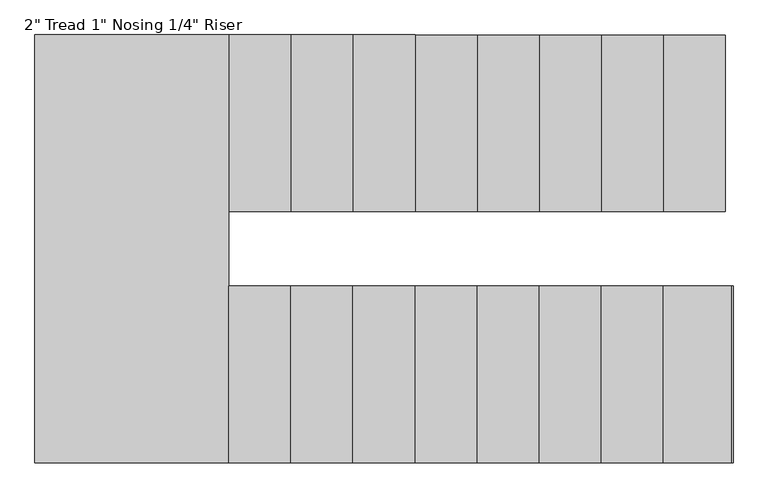
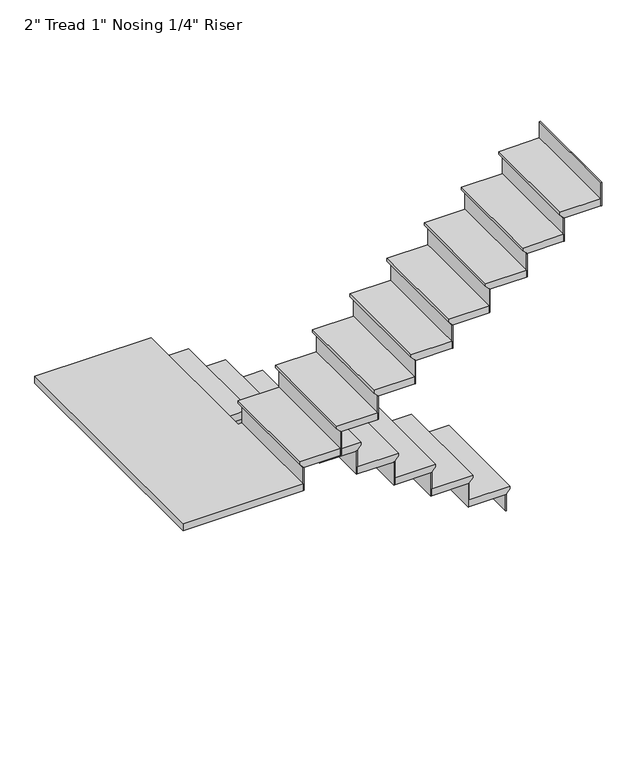
"""IFC4 building model written with IfcOpenShell, lengths in millimetres: stair flight geometry."""

from ifc_helpers import new_model, si_unit, origin, place, context, project, spatial, faceted_brep, source, transform, mapped, element, save


def stair_flight_1a1858fe(model_context):
    return source(origin(), model_context, "Body", "Brep", [
        faceted_brep([(-2118.1728655, 1192.5797121, 3196.8722222), (-2118.1728655, 1192.5797121, 3215.9222222), (-2118.1728655, 468.6797121, 3215.9222222), (-2118.1728655, 468.6797121, 3196.8722222), (-2143.5728655, 1192.5797121, 3171.4722222), (-2143.5728655, 468.6797121, 3171.4722222), (-2397.5728655, 1192.5797121, 3215.9222222), (-2397.5728655, 468.6797121, 3215.9222222), (-2143.5728655, 468.6797121, 3165.1222222), (-2397.5728655, 468.6797121, 3165.1222222), (-2397.5728655, 1192.5797121, 3165.1222222), (-2143.5728655, 1192.5797121, 3165.1222222)], [[[0, 1, 2, 3]], [[4, 0, 3, 5]], [[2, 1, 6, 7]], [[8, 9, 10, 11]], [[2, 7, 9, 8, 5, 3]], [[8, 11, 4, 5]], [[6, 1, 0, 4, 11, 10]], [[7, 6, 10, 9]]]),
        faceted_brep([(-2143.5728655, 1192.5797121, 3165.1222222), (-2143.5728655, 1192.5797121, 3048.0), (-2149.9228655, 1192.5797121, 3048.0), (-2149.9228655, 1192.5797121, 3165.1222222), (-2143.5728655, 468.6797121, 3165.1222222), (-2149.9228655, 468.6797121, 3165.1222222), (-2149.9228655, 468.6797121, 3048.0), (-2143.5728655, 468.6797121, 3048.0)], [[[0, 1, 2, 3]], [[4, 5, 6, 7]], [[1, 0, 4, 7]], [[2, 1, 7, 6]], [[3, 2, 6, 5]], [[0, 3, 5, 4]]]),
        faceted_brep([(-2397.5728655, 1192.5797121, 3333.0444444), (-2397.5728655, 1192.5797121, 3165.1222222), (-2403.9228655, 1192.5797121, 3165.1222222), (-2403.9228655, 1192.5797121, 3333.0444444), (-2397.5728655, 468.6797121, 3333.0444444), (-2403.9228655, 468.6797121, 3333.0444444), (-2403.9228655, 468.6797121, 3165.1222222), (-2397.5728655, 468.6797121, 3165.1222222)], [[[0, 1, 2, 3]], [[4, 5, 6, 7]], [[1, 0, 4, 7]], [[2, 1, 7, 6]], [[3, 2, 6, 5]], [[0, 3, 5, 4]]]),
        faceted_brep([(-2372.1728655, 468.6797121, 3383.8444444), (-2372.1728655, 1192.5797121, 3383.8444444), (-2651.5728655, 1192.5797121, 3383.8444444), (-2651.5728655, 468.6797121, 3383.8444444), (-2397.5728655, 468.6797121, 3333.0444444), (-2651.5728655, 468.6797121, 3333.0444444), (-2651.5728655, 1192.5797121, 3333.0444444), (-2397.5728655, 1192.5797121, 3333.0444444), (-2397.5728655, 468.6797121, 3339.3944444), (-2372.1728655, 468.6797121, 3364.7944444), (-2397.5728655, 1192.5797121, 3339.3944444), (-2372.1728655, 1192.5797121, 3364.7944444)], [[[0, 1, 2, 3]], [[4, 5, 6, 7]], [[0, 3, 5, 4, 8, 9]], [[4, 7, 10, 8]], [[2, 1, 11, 10, 7, 6]], [[3, 2, 6, 5]], [[11, 1, 0, 9]], [[10, 11, 9, 8]]]),
        faceted_brep([(-2651.5728655, 1192.5797121, 3500.9666667), (-2651.5728655, 1192.5797121, 3333.0444444), (-2657.9228655, 1192.5797121, 3333.0444444), (-2657.9228655, 1192.5797121, 3500.9666667), (-2651.5728655, 468.6797121, 3500.9666667), (-2657.9228655, 468.6797121, 3500.9666667), (-2657.9228655, 468.6797121, 3333.0444444), (-2651.5728655, 468.6797121, 3333.0444444)], [[[0, 1, 2, 3]], [[4, 5, 6, 7]], [[1, 0, 4, 7]], [[2, 1, 7, 6]], [[3, 2, 6, 5]], [[0, 3, 5, 4]]]),
        faceted_brep([(-2626.1728655, 468.6797121, 3551.7666667), (-2626.1728655, 1192.5797121, 3551.7666667), (-2905.5728655, 1192.5797121, 3551.7666667), (-2905.5728655, 468.6797121, 3551.7666667), (-2651.5728655, 468.6797121, 3500.9666667), (-2905.5728655, 468.6797121, 3500.9666667), (-2905.5728655, 1192.5797121, 3500.9666667), (-2651.5728655, 1192.5797121, 3500.9666667), (-2651.5728655, 468.6797121, 3507.3166667), (-2626.1728655, 468.6797121, 3532.7166667), (-2651.5728655, 1192.5797121, 3507.3166667), (-2626.1728655, 1192.5797121, 3532.7166667)], [[[0, 1, 2, 3]], [[4, 5, 6, 7]], [[0, 3, 5, 4, 8, 9]], [[4, 7, 10, 8]], [[2, 1, 11, 10, 7, 6]], [[3, 2, 6, 5]], [[11, 1, 0, 9]], [[10, 11, 9, 8]]]),
        faceted_brep([(-2905.5728655, 1192.5797121, 3668.8888889), (-2905.5728655, 1192.5797121, 3500.9666667), (-2911.9228655, 1192.5797121, 3500.9666667), (-2911.9228655, 1192.5797121, 3668.8888889), (-2905.5728655, 468.6797121, 3668.8888889), (-2911.9228655, 468.6797121, 3668.8888889), (-2911.9228655, 468.6797121, 3500.9666667), (-2905.5728655, 468.6797121, 3500.9666667)], [[[0, 1, 2, 3]], [[4, 5, 6, 7]], [[1, 0, 4, 7]], [[2, 1, 7, 6]], [[3, 2, 6, 5]], [[0, 3, 5, 4]]]),
        faceted_brep([(-2880.1728655, 468.6797121, 3719.6888889), (-2880.1728655, 1192.5797121, 3719.6888889), (-3159.5728655, 1192.5797121, 3719.6888889), (-3159.5728655, 468.6797121, 3719.6888889), (-2905.5728655, 468.6797121, 3668.8888889), (-3159.5728655, 468.6797121, 3668.8888889), (-3159.5728655, 1192.5797121, 3668.8888889), (-2905.5728655, 1192.5797121, 3668.8888889), (-2905.5728655, 468.6797121, 3675.2388889), (-2880.1728655, 468.6797121, 3700.6388889), (-2905.5728655, 1192.5797121, 3675.2388889), (-2880.1728655, 1192.5797121, 3700.6388889)], [[[0, 1, 2, 3]], [[4, 5, 6, 7]], [[0, 3, 5, 4, 8, 9]], [[4, 7, 10, 8]], [[2, 1, 11, 10, 7, 6]], [[3, 2, 6, 5]], [[11, 1, 0, 9]], [[10, 11, 9, 8]]]),
        faceted_brep([(-3159.5728655, 1192.5797121, 3836.8111111), (-3159.5728655, 1192.5797121, 3668.8888889), (-3165.9228655, 1192.5797121, 3668.8888889), (-3165.9228655, 1192.5797121, 3836.8111111), (-3159.5728655, 468.6797121, 3836.8111111), (-3165.9228655, 468.6797121, 3836.8111111), (-3165.9228655, 468.6797121, 3668.8888889), (-3159.5728655, 468.6797121, 3668.8888889)], [[[0, 1, 2, 3]], [[4, 5, 6, 7]], [[1, 0, 4, 7]], [[2, 1, 7, 6]], [[3, 2, 6, 5]], [[0, 3, 5, 4]]]),
        faceted_brep([(-3134.1728655, 468.6797121, 3887.6111111), (-3134.1728655, 1192.5797121, 3887.6111111), (-3413.5728655, 1192.5797121, 3887.6111111), (-3413.5728655, 468.6797121, 3887.6111111), (-3159.5728655, 468.6797121, 3836.8111111), (-3413.5728655, 468.6797121, 3836.8111111), (-3413.5728655, 1192.5797121, 3836.8111111), (-3159.5728655, 1192.5797121, 3836.8111111), (-3159.5728655, 468.6797121, 3843.1611111), (-3134.1728655, 468.6797121, 3868.5611111), (-3159.5728655, 1192.5797121, 3843.1611111), (-3134.1728655, 1192.5797121, 3868.5611111)], [[[0, 1, 2, 3]], [[4, 5, 6, 7]], [[0, 3, 5, 4, 8, 9]], [[4, 7, 10, 8]], [[2, 1, 11, 10, 7, 6]], [[3, 2, 6, 5]], [[11, 1, 0, 9]], [[10, 11, 9, 8]]]),
        faceted_brep([(-3413.5728655, 1192.5797121, 4004.7333333), (-3413.5728655, 1192.5797121, 3836.8111111), (-3419.9228655, 1192.5797121, 3836.8111111), (-3419.9228655, 1192.5797121, 4004.7333333), (-3413.5728655, 468.6797121, 4004.7333333), (-3419.9228655, 468.6797121, 4004.7333333), (-3419.9228655, 468.6797121, 3836.8111111), (-3413.5728655, 468.6797121, 3836.8111111)], [[[0, 1, 2, 3]], [[4, 5, 6, 7]], [[1, 0, 4, 7]], [[2, 1, 7, 6]], [[3, 2, 6, 5]], [[0, 3, 5, 4]]]),
        faceted_brep([(-3388.1728655, 468.6797121, 4055.5333333), (-3388.1728655, 1192.5797121, 4055.5333333), (-3667.5728655, 1192.5797121, 4055.5333333), (-3667.5728655, 468.6797121, 4055.5333333), (-3413.5728655, 468.6797121, 4004.7333333), (-3667.5728655, 468.6797121, 4004.7333333), (-3667.5728655, 1192.5797121, 4004.7333333), (-3413.5728655, 1192.5797121, 4004.7333333), (-3413.5728655, 468.6797121, 4011.0833333), (-3388.1728655, 468.6797121, 4036.4833333), (-3413.5728655, 1192.5797121, 4011.0833333), (-3388.1728655, 1192.5797121, 4036.4833333)], [[[0, 1, 2, 3]], [[4, 5, 6, 7]], [[0, 3, 5, 4, 8, 9]], [[4, 7, 10, 8]], [[2, 1, 11, 10, 7, 6]], [[3, 2, 6, 5]], [[11, 1, 0, 9]], [[10, 11, 9, 8]]]),
        faceted_brep([(-3667.5728655, 1192.5797121, 4172.6555556), (-3667.5728655, 1192.5797121, 4004.7333333), (-3673.9228655, 1192.5797121, 4004.7333333), (-3673.9228655, 1192.5797121, 4172.6555556), (-3667.5728655, 468.6797121, 4172.6555556), (-3673.9228655, 468.6797121, 4172.6555556), (-3673.9228655, 468.6797121, 4004.7333333), (-3667.5728655, 468.6797121, 4004.7333333)], [[[0, 1, 2, 3]], [[4, 5, 6, 7]], [[1, 0, 4, 7]], [[2, 1, 7, 6]], [[3, 2, 6, 5]], [[0, 3, 5, 4]]]),
        faceted_brep([(-3642.1728655, 468.6797121, 4223.4555556), (-3642.1728655, 1192.5797121, 4223.4555556), (-3921.5728655, 1192.5797121, 4223.4555556), (-3921.5728655, 468.6797121, 4223.4555556), (-3667.5728655, 468.6797121, 4172.6555556), (-3921.5728655, 468.6797121, 4172.6555556), (-3921.5728655, 1192.5797121, 4172.6555556), (-3667.5728655, 1192.5797121, 4172.6555556), (-3667.5728655, 468.6797121, 4179.0055556), (-3642.1728655, 468.6797121, 4204.4055556), (-3667.5728655, 1192.5797121, 4179.0055556), (-3642.1728655, 1192.5797121, 4204.4055556)], [[[0, 1, 2, 3]], [[4, 5, 6, 7]], [[0, 3, 5, 4, 8, 9]], [[4, 7, 10, 8]], [[2, 1, 11, 10, 7, 6]], [[3, 2, 6, 5]], [[11, 1, 0, 9]], [[10, 11, 9, 8]]]),
        faceted_brep([(-3921.5728655, 1192.5797121, 4340.5777778), (-3921.5728655, 1192.5797121, 4172.6555556), (-3927.9228655, 1192.5797121, 4172.6555556), (-3927.9228655, 1192.5797121, 4340.5777778), (-3921.5728655, 468.6797121, 4340.5777778), (-3927.9228655, 468.6797121, 4340.5777778), (-3927.9228655, 468.6797121, 4172.6555556), (-3921.5728655, 468.6797121, 4172.6555556)], [[[0, 1, 2, 3]], [[4, 5, 6, 7]], [[1, 0, 4, 7]], [[2, 1, 7, 6]], [[3, 2, 6, 5]], [[0, 3, 5, 4]]]),
        faceted_brep([(-3896.1728655, 468.6797121, 4391.3777778), (-3896.1728655, 1192.5797121, 4391.3777778), (-4175.5728655, 1192.5797121, 4391.3777778), (-4175.5728655, 468.6797121, 4391.3777778), (-3921.5728655, 468.6797121, 4340.5777778), (-4175.5728655, 468.6797121, 4340.5777778), (-4175.5728655, 1192.5797121, 4340.5777778), (-3921.5728655, 1192.5797121, 4340.5777778), (-3921.5728655, 468.6797121, 4346.9277778), (-3896.1728655, 468.6797121, 4372.3277778), (-3921.5728655, 1192.5797121, 4346.9277778), (-3896.1728655, 1192.5797121, 4372.3277778)], [[[0, 1, 2, 3]], [[4, 5, 6, 7]], [[0, 3, 5, 4, 8, 9]], [[4, 7, 10, 8]], [[2, 1, 11, 10, 7, 6]], [[3, 2, 6, 5]], [[11, 1, 0, 9]], [[10, 11, 9, 8]]]),
        faceted_brep([(-4175.5728655, 1192.5797121, 4508.5), (-4175.5728655, 1192.5797121, 4340.5777778), (-4181.9228655, 1192.5797121, 4340.5777778), (-4181.9228655, 1192.5797121, 4508.5), (-4175.5728655, 468.6797121, 4508.5), (-4181.9228655, 468.6797121, 4508.5), (-4181.9228655, 468.6797121, 4340.5777778), (-4175.5728655, 468.6797121, 4340.5777778)], [[[0, 1, 2, 3]], [[4, 5, 6, 7]], [[1, 0, 4, 7]], [[2, 1, 7, 6]], [[3, 2, 6, 5]], [[0, 3, 5, 4]]]),
        faceted_brep([(-4124.7728655, 163.8797121, 4559.3), (-4150.1728655, 163.8797121, 4559.3), (-4150.1728655, 1192.5797121, 4559.3), (-4943.9394105, 1192.5797121, 4559.3), (-4943.9394105, -560.0202879, 4559.3), (-4124.7728655, -560.0202879, 4559.3), (-4150.1728655, 163.8797121, 4508.5), (-4124.7728655, 163.8797121, 4508.5), (-4124.7728655, -560.0202879, 4508.5), (-4943.9394105, -560.0202879, 4508.5), (-4943.9394105, 1192.5797121, 4508.5), (-4175.5728655, 1192.5797121, 4508.5), (-4175.5728655, 468.6797121, 4508.5), (-4150.1728655, 468.6797121, 4508.5), (-4150.1728655, 468.6797121, 4540.25), (-4150.1728655, 1192.5797121, 4540.25), (-4175.5728655, 468.6797121, 4514.85), (-4175.5728655, 1192.5797121, 4514.85)], [[[0, 1, 2, 3, 4, 5]], [[6, 7, 8, 9, 10, 11, 12, 13]], [[1, 0, 7, 6]], [[2, 1, 6, 13, 14, 15]], [[13, 12, 16, 14]], [[12, 11, 17, 16]], [[3, 2, 15, 17, 11, 10]], [[4, 3, 10, 9]], [[5, 4, 9, 8]], [[0, 5, 8, 7]], [[17, 15, 14, 16]]]),
        faceted_brep([(-4124.7728655, -560.0202879, 4676.4222222), (-4124.7728655, -560.0202879, 4508.5), (-4118.4228655, -560.0202879, 4508.5), (-4118.4228655, -560.0202879, 4676.4222222), (-4124.7728655, 163.8797121, 4676.4222222), (-4118.4228655, 163.8797121, 4676.4222222), (-4118.4228655, 163.8797121, 4508.5), (-4124.7728655, 163.8797121, 4508.5)], [[[0, 1, 2, 3]], [[4, 5, 6, 7]], [[1, 0, 4, 7]], [[2, 1, 7, 6]], [[3, 2, 6, 5]], [[0, 3, 5, 4]]]),
        faceted_brep([(-4150.1728655, 163.8797121, 4727.2222222), (-4150.1728655, -560.0202879, 4727.2222222), (-3870.7728655, -560.0202879, 4727.2222222), (-3870.7728655, 163.8797121, 4727.2222222), (-4124.7728655, 163.8797121, 4676.4222222), (-3870.7728655, 163.8797121, 4676.4222222), (-3870.7728655, -560.0202879, 4676.4222222), (-4124.7728655, -560.0202879, 4676.4222222), (-4124.7728655, 163.8797121, 4682.7722222), (-4150.1728655, 163.8797121, 4708.1722222), (-4124.7728655, -560.0202879, 4682.7722222), (-4150.1728655, -560.0202879, 4708.1722222)], [[[0, 1, 2, 3]], [[4, 5, 6, 7]], [[0, 3, 5, 4, 8, 9]], [[4, 7, 10, 8]], [[2, 1, 11, 10, 7, 6]], [[3, 2, 6, 5]], [[11, 1, 0, 9]], [[10, 11, 9, 8]]]),
        faceted_brep([(-3870.7728655, -560.0202879, 4844.3444444), (-3870.7728655, -560.0202879, 4676.4222222), (-3864.4228655, -560.0202879, 4676.4222222), (-3864.4228655, -560.0202879, 4844.3444444), (-3870.7728655, 163.8797121, 4844.3444444), (-3864.4228655, 163.8797121, 4844.3444444), (-3864.4228655, 163.8797121, 4676.4222222), (-3870.7728655, 163.8797121, 4676.4222222)], [[[0, 1, 2, 3]], [[4, 5, 6, 7]], [[1, 0, 4, 7]], [[2, 1, 7, 6]], [[3, 2, 6, 5]], [[0, 3, 5, 4]]]),
        faceted_brep([(-3896.1728655, 163.8797121, 4895.1444444), (-3896.1728655, -560.0202879, 4895.1444444), (-3616.7728655, -560.0202879, 4895.1444444), (-3616.7728655, 163.8797121, 4895.1444444), (-3870.7728655, 163.8797121, 4844.3444444), (-3616.7728655, 163.8797121, 4844.3444444), (-3616.7728655, -560.0202879, 4844.3444444), (-3870.7728655, -560.0202879, 4844.3444444), (-3870.7728655, 163.8797121, 4850.6944444), (-3896.1728655, 163.8797121, 4876.0944444), (-3870.7728655, -560.0202879, 4850.6944444), (-3896.1728655, -560.0202879, 4876.0944444)], [[[0, 1, 2, 3]], [[4, 5, 6, 7]], [[0, 3, 5, 4, 8, 9]], [[4, 7, 10, 8]], [[2, 1, 11, 10, 7, 6]], [[3, 2, 6, 5]], [[11, 1, 0, 9]], [[10, 11, 9, 8]]]),
        faceted_brep([(-3616.7728655, -560.0202879, 5012.2666667), (-3616.7728655, -560.0202879, 4844.3444444), (-3610.4228655, -560.0202879, 4844.3444444), (-3610.4228655, -560.0202879, 5012.2666667), (-3616.7728655, 163.8797121, 5012.2666667), (-3610.4228655, 163.8797121, 5012.2666667), (-3610.4228655, 163.8797121, 4844.3444444), (-3616.7728655, 163.8797121, 4844.3444444)], [[[0, 1, 2, 3]], [[4, 5, 6, 7]], [[1, 0, 4, 7]], [[2, 1, 7, 6]], [[3, 2, 6, 5]], [[0, 3, 5, 4]]]),
        faceted_brep([(-3642.1728655, 163.8797121, 5063.0666667), (-3642.1728655, -560.0202879, 5063.0666667), (-3362.7728655, -560.0202879, 5063.0666667), (-3362.7728655, 163.8797121, 5063.0666667), (-3616.7728655, 163.8797121, 5012.2666667), (-3362.7728655, 163.8797121, 5012.2666667), (-3362.7728655, -560.0202879, 5012.2666667), (-3616.7728655, -560.0202879, 5012.2666667), (-3616.7728655, 163.8797121, 5018.6166667), (-3642.1728655, 163.8797121, 5044.0166667), (-3616.7728655, -560.0202879, 5018.6166667), (-3642.1728655, -560.0202879, 5044.0166667)], [[[0, 1, 2, 3]], [[4, 5, 6, 7]], [[0, 3, 5, 4, 8, 9]], [[4, 7, 10, 8]], [[2, 1, 11, 10, 7, 6]], [[3, 2, 6, 5]], [[11, 1, 0, 9]], [[10, 11, 9, 8]]]),
        faceted_brep([(-3362.7728655, -560.0202879, 5180.1888889), (-3362.7728655, -560.0202879, 5012.2666667), (-3356.4228655, -560.0202879, 5012.2666667), (-3356.4228655, -560.0202879, 5180.1888889), (-3362.7728655, 163.8797121, 5180.1888889), (-3356.4228655, 163.8797121, 5180.1888889), (-3356.4228655, 163.8797121, 5012.2666667), (-3362.7728655, 163.8797121, 5012.2666667)], [[[0, 1, 2, 3]], [[4, 5, 6, 7]], [[1, 0, 4, 7]], [[2, 1, 7, 6]], [[3, 2, 6, 5]], [[0, 3, 5, 4]]]),
        faceted_brep([(-3388.1728655, 163.8797121, 5230.9888889), (-3388.1728655, -560.0202879, 5230.9888889), (-3108.7728655, -560.0202879, 5230.9888889), (-3108.7728655, 163.8797121, 5230.9888889), (-3362.7728655, 163.8797121, 5180.1888889), (-3108.7728655, 163.8797121, 5180.1888889), (-3108.7728655, -560.0202879, 5180.1888889), (-3362.7728655, -560.0202879, 5180.1888889), (-3362.7728655, 163.8797121, 5186.5388889), (-3388.1728655, 163.8797121, 5211.9388889), (-3362.7728655, -560.0202879, 5186.5388889), (-3388.1728655, -560.0202879, 5211.9388889)], [[[0, 1, 2, 3]], [[4, 5, 6, 7]], [[0, 3, 5, 4, 8, 9]], [[4, 7, 10, 8]], [[2, 1, 11, 10, 7, 6]], [[3, 2, 6, 5]], [[11, 1, 0, 9]], [[10, 11, 9, 8]]]),
        faceted_brep([(-3108.7728655, -560.0202879, 5348.1111111), (-3108.7728655, -560.0202879, 5180.1888889), (-3102.4228655, -560.0202879, 5180.1888889), (-3102.4228655, -560.0202879, 5348.1111111), (-3108.7728655, 163.8797121, 5348.1111111), (-3102.4228655, 163.8797121, 5348.1111111), (-3102.4228655, 163.8797121, 5180.1888889), (-3108.7728655, 163.8797121, 5180.1888889)], [[[0, 1, 2, 3]], [[4, 5, 6, 7]], [[1, 0, 4, 7]], [[2, 1, 7, 6]], [[3, 2, 6, 5]], [[0, 3, 5, 4]]]),
        faceted_brep([(-3134.1728655, 163.8797121, 5398.9111111), (-3134.1728655, -560.0202879, 5398.9111111), (-2854.7728655, -560.0202879, 5398.9111111), (-2854.7728655, 163.8797121, 5398.9111111), (-3108.7728655, 163.8797121, 5348.1111111), (-2854.7728655, 163.8797121, 5348.1111111), (-2854.7728655, -560.0202879, 5348.1111111), (-3108.7728655, -560.0202879, 5348.1111111), (-3108.7728655, 163.8797121, 5354.4611111), (-3134.1728655, 163.8797121, 5379.8611111), (-3108.7728655, -560.0202879, 5354.4611111), (-3134.1728655, -560.0202879, 5379.8611111)], [[[0, 1, 2, 3]], [[4, 5, 6, 7]], [[0, 3, 5, 4, 8, 9]], [[4, 7, 10, 8]], [[2, 1, 11, 10, 7, 6]], [[3, 2, 6, 5]], [[11, 1, 0, 9]], [[10, 11, 9, 8]]]),
        faceted_brep([(-2854.7728655, -560.0202879, 5516.0333333), (-2854.7728655, -560.0202879, 5348.1111111), (-2848.4228655, -560.0202879, 5348.1111111), (-2848.4228655, -560.0202879, 5516.0333333), (-2854.7728655, 163.8797121, 5516.0333333), (-2848.4228655, 163.8797121, 5516.0333333), (-2848.4228655, 163.8797121, 5348.1111111), (-2854.7728655, 163.8797121, 5348.1111111)], [[[0, 1, 2, 3]], [[4, 5, 6, 7]], [[1, 0, 4, 7]], [[2, 1, 7, 6]], [[3, 2, 6, 5]], [[0, 3, 5, 4]]]),
        faceted_brep([(-2880.1728655, 163.8797121, 5566.8333333), (-2880.1728655, -560.0202879, 5566.8333333), (-2600.7728655, -560.0202879, 5566.8333333), (-2600.7728655, 163.8797121, 5566.8333333), (-2854.7728655, 163.8797121, 5516.0333333), (-2600.7728655, 163.8797121, 5516.0333333), (-2600.7728655, -560.0202879, 5516.0333333), (-2854.7728655, -560.0202879, 5516.0333333), (-2854.7728655, 163.8797121, 5522.3833333), (-2880.1728655, 163.8797121, 5547.7833333), (-2854.7728655, -560.0202879, 5522.3833333), (-2880.1728655, -560.0202879, 5547.7833333)], [[[0, 1, 2, 3]], [[4, 5, 6, 7]], [[0, 3, 5, 4, 8, 9]], [[4, 7, 10, 8]], [[2, 1, 11, 10, 7, 6]], [[3, 2, 6, 5]], [[11, 1, 0, 9]], [[10, 11, 9, 8]]]),
        faceted_brep([(-2600.7728655, -560.0202879, 5683.9555556), (-2600.7728655, -560.0202879, 5516.0333333), (-2594.4228655, -560.0202879, 5516.0333333), (-2594.4228655, -560.0202879, 5683.9555556), (-2600.7728655, 163.8797121, 5683.9555556), (-2594.4228655, 163.8797121, 5683.9555556), (-2594.4228655, 163.8797121, 5516.0333333), (-2600.7728655, 163.8797121, 5516.0333333)], [[[0, 1, 2, 3]], [[4, 5, 6, 7]], [[1, 0, 4, 7]], [[2, 1, 7, 6]], [[3, 2, 6, 5]], [[0, 3, 5, 4]]]),
        faceted_brep([(-2626.1728655, 163.8797121, 5734.7555556), (-2626.1728655, -560.0202879, 5734.7555556), (-2346.7728655, -560.0202879, 5734.7555556), (-2346.7728655, 163.8797121, 5734.7555556), (-2600.7728655, 163.8797121, 5683.9555556), (-2346.7728655, 163.8797121, 5683.9555556), (-2346.7728655, -560.0202879, 5683.9555556), (-2600.7728655, -560.0202879, 5683.9555556), (-2600.7728655, 163.8797121, 5690.3055556), (-2626.1728655, 163.8797121, 5715.7055556), (-2600.7728655, -560.0202879, 5690.3055556), (-2626.1728655, -560.0202879, 5715.7055556)], [[[0, 1, 2, 3]], [[4, 5, 6, 7]], [[0, 3, 5, 4, 8, 9]], [[4, 7, 10, 8]], [[2, 1, 11, 10, 7, 6]], [[3, 2, 6, 5]], [[11, 1, 0, 9]], [[10, 11, 9, 8]]]),
        faceted_brep([(-2346.7728655, -560.0202879, 5851.8777778), (-2346.7728655, -560.0202879, 5683.9555556), (-2340.4228655, -560.0202879, 5683.9555556), (-2340.4228655, -560.0202879, 5851.8777778), (-2346.7728655, 163.8797121, 5851.8777778), (-2340.4228655, 163.8797121, 5851.8777778), (-2340.4228655, 163.8797121, 5683.9555556), (-2346.7728655, 163.8797121, 5683.9555556)], [[[0, 1, 2, 3]], [[4, 5, 6, 7]], [[1, 0, 4, 7]], [[2, 1, 7, 6]], [[3, 2, 6, 5]], [[0, 3, 5, 4]]]),
        faceted_brep([(-2092.7728655, -560.0202879, 6019.8), (-2092.7728655, -560.0202879, 5851.8777778), (-2086.4228655, -560.0202879, 5851.8777778), (-2086.4228655, -560.0202879, 6019.8), (-2092.7728655, 163.8797121, 6019.8), (-2086.4228655, 163.8797121, 6019.8), (-2086.4228655, 163.8797121, 5851.8777778), (-2092.7728655, 163.8797121, 5851.8777778)], [[[0, 1, 2, 3]], [[4, 5, 6, 7]], [[1, 0, 4, 7]], [[2, 1, 7, 6]], [[3, 2, 6, 5]], [[0, 3, 5, 4]]]),
        faceted_brep([(-2372.1728655, 163.8797121, 5902.6777778), (-2372.1728655, -560.0202879, 5902.6777778), (-2092.7728655, -560.0202879, 5902.6777778), (-2092.7728655, 163.8797121, 5902.6777778), (-2346.7728655, 163.8797121, 5851.8777778), (-2092.7728655, 163.8797121, 5851.8777778), (-2092.7728655, -560.0202879, 5851.8777778), (-2346.7728655, -560.0202879, 5851.8777778), (-2346.7728655, 163.8797121, 5858.2277778), (-2372.1728655, 163.8797121, 5883.6277778), (-2346.7728655, -560.0202879, 5858.2277778), (-2372.1728655, -560.0202879, 5883.6277778)], [[[0, 1, 2, 3]], [[4, 5, 6, 7]], [[0, 3, 5, 4, 8, 9]], [[4, 7, 10, 8]], [[2, 1, 11, 10, 7, 6]], [[3, 2, 6, 5]], [[11, 1, 0, 9]], [[10, 11, 9, 8]]]),
    ])


if __name__ == "__main__":
    model = new_model("IFC4")
    model_context = context("Model", 3, world=origin())
    ifc_project = project(units=[si_unit("LENGTHUNIT", "METRE", prefix="MILLI")], contexts=[model_context])
    site = spatial("IfcSite", under=ifc_project)
    building = spatial("IfcBuilding", under=site)
    placement = place(None, origin())
    stair_flight_shape = stair_flight_1a1858fe(model_context)
    element("IfcStairFlight", 1, ObjectType="2\" Tread 1\" Nosing 1/4\" Riser", at=placement, inside=building, context=model_context, shape_type="MappedRepresentation", body=[
        mapped(stair_flight_shape, transform((0.0, 0.0, 0.0), x_axis=(1.0, 0.0, 0.0), y_axis=(0.0, 1.0, 0.0), z_axis=(0.0, 0.0, 1.0))),
    ])
    save(model, "model.ifc")
